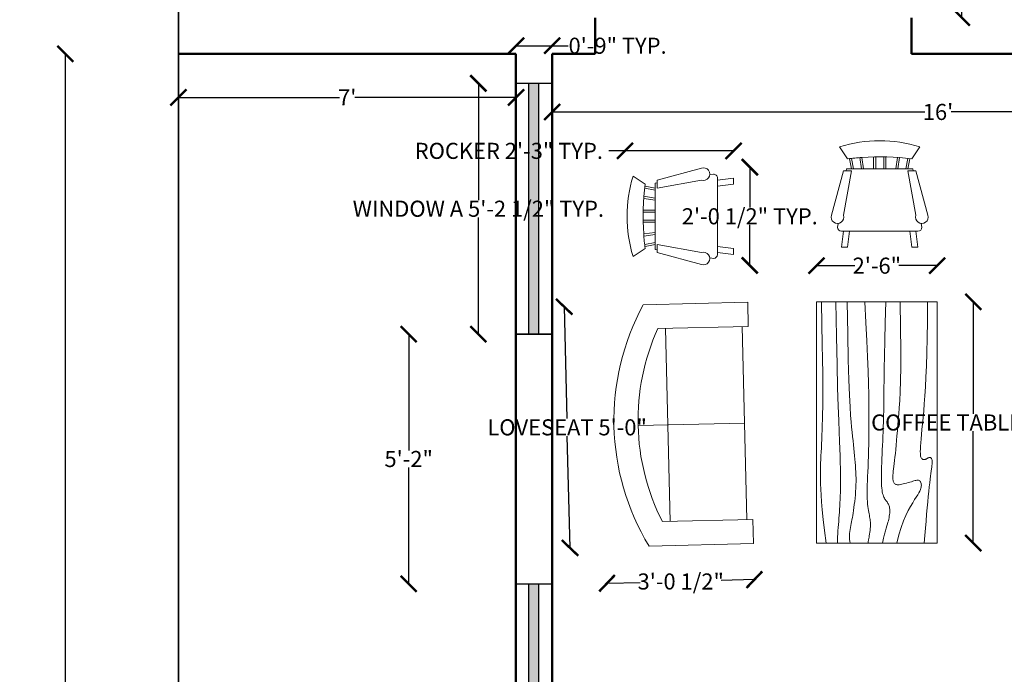
# Model space of a CAD drawing. Units: inches. Extents: x 2466 to 2986, y -30 to 527.
# Tile 2 of 5: x 2466 to 2711, y 190 to 353. Entities that reach past the tile are written whole.
import ezdxf

# ---------------------------------------------------------------- set-up
doc = ezdxf.new("R2010")
doc.units = ezdxf.units.IN
for name, color, linetype, lineweight in [('A-ANNO-DIMS', 2, 'Continuous', 18), ('A-GLAZ', 4, 'Continuous', 25), ('C-PROP', 40, 'Continuous', 35), ('furniture', 6, 'Continuous', 18), ('walls', 40, 'Continuous', 50)]:
    doc.layers.add(name, color=color, linetype=linetype, lineweight=lineweight)
doc.styles.get("Standard").update_dxf_attribs({"font": 'arial.ttf'})
doc.dimstyles.get("Standard").update_dxf_attribs({"dimtxt": 4, "dimasz": 4, "dimexe": 0.18, "dimexo": 0.0625, "dimgap": 0.09, "dimtad": 0, "dimtih": 1, "dimtoh": 1, "dimzin": 0, "dimdsep": 46, "dimlunit": 3, "dimtxsty": 'Standard', "dimblk": 'ARCHTICK', "dimcen": 0.09, "dimse1": 1, "dimse2": 1, "dimclrd": 3, "dimclrt": 2, "dimadec": 0, "dimazin": 0, "dimtfac": 1, "dimtofl": 0, "dimtmove": 0, "dimatfit": 3, "dimfxl": 1, "dimtolj": 1, "dimtzin": 0, "dimarcsym": 0})

# ---------------------------------------------------------------- blocks, each defined once
blk = doc.blocks.new('Sofa - Roundback Loveseat 5 ft.')
for p, q in [((0, -32.44198), (0, -5.99998)), ((-24, -33.99998), (-24, -11.46958)), ((24.00004, -33.99998), (24.00004, -11.46958)), ((-23.9998, -13.38178), (23.99986, -13.38178)), ((-24, -32.44198), (24.00004, -32.44198))]:
    blk.add_line(p, q)
for points in [[(-24, -33.99998), (-30, -33.99998), (-30, -7.99998)], [(30.00004, -7.99998), (30.00004, -33.99998), (24.00004, -33.99998)]]:
    blk.add_lwpolyline(points)
for centre, radius, start, end in [((0, -60.24998), 60.24998, 60.13715, 119.8628), ((0, -61.38438), 55.38444, 64.32083, 115.6792)]:
    blk.add_arc(centre, radius, start, end)
blk = doc.blocks.new('Table - Rectangular Woodgrain 60 x 30 in.')
for p, q in [((0, 0), (0, -30)), ((60, 0), (0, 0)), ((60, -30), (60, 0)), ((0, -30), (60, -30))]:
    blk.add_line(p, q)
for points in [[(0, -2.4), (4.8155, -2.418), (9.0302, -2.4688), (12.709, -2.5477), (15.9167, -2.65), (18.7181, -2.7711), (21.1781, -2.9063), (23.3616, -3.0508), (25.3333, -3.2), (27.1477, -3.3495), (28.8172, -3.4958), (30.3437, -3.636), (31.7291, -3.7667), (32.9756, -3.8849), (34.0849, -3.9875), (35.059, -4.0714), (35.9, -4.1334), (36.6114, -4.1711), (37.2041, -4.1854), (37.6906, -4.1779), (38.0833, -4.15), (38.3948, -4.1034), (38.6375, -4.0396), (38.8239, -3.9602), (38.9666, -3.8667), (39.0764, -3.7608), (39.1573, -3.6448), (39.2116, -3.521), (39.2416, -3.3917), (39.2498, -3.2593), (39.2385, -3.1261), (39.21, -2.9944), (39.1666, -2.8667), (39.111, -2.7447), (39.0468, -2.6281), (38.978, -2.5163), (38.9083, -2.4083), (38.8418, -2.3035), (38.7823, -2.201), (38.7337, -2.1001), (38.7, -2), (38.6844, -1.9003), (38.6875, -1.8021), (38.7094, -1.707), (38.75, -1.6167), (38.8094, -1.5326), (38.8875, -1.4563), (38.9844, -1.3893), (39.1, -1.3333), (39.2351, -1.2896), (39.3937, -1.2583), (39.5804, -1.2396), (39.8, -1.2333), (40.057, -1.2396), (40.3562, -1.2583), (40.7023, -1.2896), (41.1, -1.3333), (41.5547, -1.3895), (42.0755, -1.4573), (42.6721, -1.5361), (43.3542, -1.625), (44.1316, -1.7233), (45.014, -1.8302), (46.0114, -1.9449), (47.1333, -2.0667), (48.3862, -2.1947), (49.7625, -2.3281), (51.2513, -2.4663), (52.8416, -2.6083), (54.5226, -2.7535), (56.2833, -2.9011), (58.1127, -3.0501), (60, -3.2)], [(0, -9.2), (6.5759, -9.0858), (11.9385, -9.0365), (16.2527, -9.0418), (19.6833, -9.0917), (22.3952, -9.1759), (24.5531, -9.2844), (26.322, -9.4069), (27.8666, -9.5333), (29.3241, -9.6553), (30.7203, -9.7719), (32.0532, -9.8837), (33.3208, -9.9917), (34.5213, -10.0965), (35.6526, -10.199), (36.7128, -10.2999), (37.7, -10.4), (38.6129, -10.4996), (39.4531, -10.5969), (40.223, -10.6895), (40.925, -10.775), (41.5613, -10.8512), (42.1344, -10.9156), (42.6465, -10.966), (43.1, -11), (43.4976, -11.0158), (43.8437, -11.0136), (44.143, -10.9942), (44.4, -10.9583), (44.6195, -10.9069), (44.8062, -10.8406), (44.9648, -10.7603), (45.1, -10.6667), (45.2155, -10.5598), (45.3114, -10.4365), (45.3871, -10.2929), (45.4416, -10.125), (45.4743, -9.929), (45.4844, -9.7011), (45.4709, -9.4371), (45.4333, -9.1333), (45.3716, -8.7883), (45.2896, -8.4104), (45.1919, -8.0107), (45.0833, -7.6), (44.9685, -7.1893), (44.8521, -6.7896), (44.7388, -6.4117), (44.6333, -6.0667), (44.54, -5.7628), (44.4614, -5.4979), (44.4001, -5.2675), (44.3583, -5.0667), (44.3384, -4.8909), (44.3427, -4.7354), (44.3736, -4.5956), (44.4333, -4.4667), (44.5236, -4.3453), (44.6427, -4.2333), (44.7884, -4.1339), (44.9583, -4.05), (45.1501, -3.9849), (45.3614, -3.9417), (45.59, -3.9234), (45.8333, -3.9333), (46.0915, -3.9749), (46.3734, -4.0531), (46.6906, -4.1736), (47.0542, -4.3417), (47.4756, -4.5629), (47.9661, -4.8427), (48.5372, -5.1866), (49.2, -5.6), (49.9676, -6.0844), (50.8594, -6.625), (51.8965, -7.2031), (53.1, -7.8), (54.491, -8.3969), (56.0906, -8.975), (57.9199, -9.5156), (60, -10)], [(0, -12.8), (5.1847, -12.9322), (9.6213, -13.0323), (13.3963, -13.1059), (16.5958, -13.1583), (19.3063, -13.1952), (21.614, -13.2219), (23.6054, -13.2439), (25.3666, -13.2667), (26.9728, -13.2947), (28.4531, -13.3281), (29.8256, -13.3663), (31.1083, -13.4083), (32.3191, -13.4535), (33.476, -13.501), (34.597, -13.5501), (35.7, -13.6), (36.7984, -13.6497), (37.8875, -13.6979), (38.9578, -13.743), (40, -13.7833), (41.0047, -13.8174), (41.9625, -13.8438), (42.864, -13.8607), (43.7, -13.8667), (44.4631, -13.8604), (45.1552, -13.8417), (45.7801, -13.8104), (46.3416, -13.7667), (46.8439, -13.7104), (47.2906, -13.6417), (47.6858, -13.5604), (48.0333, -13.4667), (48.3375, -13.3608), (48.6042, -13.2448), (48.8396, -13.121), (49.05, -12.9917), (49.2417, -12.8593), (49.4208, -12.7261), (49.5937, -12.5944), (49.7667, -12.4667), (49.9452, -12.3451), (50.1323, -12.2313), (50.3303, -12.1268), (50.5416, -12.0333), (50.7686, -11.9524), (51.0135, -11.8854), (51.2788, -11.8341), (51.5666, -11.8), (51.8785, -11.7843), (52.2116, -11.7865), (52.562, -11.8059), (52.926, -11.8417), (53.2998, -11.8931), (53.6795, -11.9594), (54.0614, -12.0397), (54.4416, -12.1333), (54.8223, -12.2401), (55.2293, -12.3625), (55.6942, -12.5037), (56.2489, -12.6667), (56.9251, -12.8547), (57.7545, -13.0708), (58.7689, -13.3182), (60, -13.6)], [(0, -18), (5.124, -17.7273), (9.6609, -17.5057), (13.6705, -17.3303), (17.2125, -17.1958), (20.3467, -17.0973), (23.1328, -17.0297), (25.6307, -16.9878), (27.9, -16.9667), (29.9928, -16.9617), (31.9302, -16.9703), (33.7254, -16.9907), (35.3917, -17.0208), (36.9423, -17.0588), (38.3906, -17.1026), (39.7499, -17.1503), (41.0333, -17.2), (42.2519, -17.2496), (43.4073, -17.2969), (44.4986, -17.3395), (45.525, -17.375), (46.4858, -17.4012), (47.3802, -17.4156), (48.2074, -17.416), (48.9667, -17.4), (49.6583, -17.3662), (50.2872, -17.3167), (50.8595, -17.2547), (51.3812, -17.1833), (51.8584, -17.1057), (52.2971, -17.025), (52.7034, -16.9443), (53.0833, -16.8667), (53.443, -16.7951), (53.789, -16.7313), (54.128, -16.6768), (54.4666, -16.6334), (54.8115, -16.6024), (55.1693, -16.5854), (55.5465, -16.5841), (55.95, -16.6), (56.3828, -16.6337), (56.8346, -16.6823), (57.2915, -16.7418), (57.7396, -16.8084), (58.165, -16.878), (58.5539, -16.9469), (58.8924, -17.0111), (59.1666, -17.0667), (59.3679, -17.1107), (59.5078, -17.1438), (59.6032, -17.1675), (59.6708, -17.1833), (59.7275, -17.193), (59.7901, -17.1979), (59.8753, -17.1998), (60, -17.2)], [(0, -22.4), (8.0098, -22.2501), (14.4094, -22.1011), (19.4168, -21.9535), (23.25, -21.8083), (26.1269, -21.6663), (28.2656, -21.5281), (29.884, -21.3947), (31.2, -21.2667), (32.3967, -21.1448), (33.5172, -21.0292), (34.5697, -20.9198), (35.5625, -20.8167), (36.5037, -20.7198), (37.4015, -20.6292), (38.2642, -20.5448), (39.1, -20.4667), (39.9164, -20.3951), (40.7187, -20.3313), (41.5117, -20.2768), (42.3, -20.2333), (43.0883, -20.2024), (43.8812, -20.1854), (44.6836, -20.1841), (45.5, -20.2), (46.3328, -20.234), (47.1747, -20.2844), (48.0163, -20.3488), (48.8479, -20.425), (49.66, -20.5106), (50.4429, -20.6031), (51.1872, -20.7004), (51.8833, -20.8), (52.5246, -20.8999), (53.1166, -20.9995), (53.6681, -21.0983), (54.1875, -21.1958), (54.6834, -21.2919), (55.1646, -21.3859), (55.6394, -21.4777), (56.1167, -21.5667), (56.6028, -21.6515), (57.0961, -21.7266), (57.5929, -21.7852), (58.0896, -21.8208), (58.5823, -21.8268), (59.0674, -21.7964), (59.5412, -21.723), (60, -21.6)], [(0, -25.2), (8.6355, -25.0504), (15.7026, -24.9031), (21.4049, -24.7606), (25.9458, -24.625), (29.529, -24.4988), (32.3578, -24.3844), (34.6359, -24.284), (36.5667, -24.2), (38.3213, -24.1341), (39.9417, -24.0854), (41.437, -24.0523), (42.8167, -24.0333), (44.0901, -24.0268), (45.2667, -24.0313), (46.3557, -24.0451), (47.3667, -24.0667), (48.309, -24.0947), (49.1928, -24.1287), (50.0284, -24.168), (50.826, -24.2125), (51.5959, -24.2617), (52.3483, -24.3151), (53.0935, -24.3725), (53.8417, -24.4334), (54.6009, -24.497), (55.3699, -24.561), (56.1454, -24.6226), (56.9239, -24.6792), (57.7021, -24.7279), (58.4764, -24.7662), (59.2435, -24.7911), (60, -24.8)], [(0, -28.8), (5.6867, -28.6681), (10.45, -28.5698), (14.407, -28.5012), (17.675, -28.4584), (20.3711, -28.4374), (22.6125, -28.4344), (24.5164, -28.4455), (26.2, -28.4667), (27.762, -28.4947), (29.2276, -28.5281), (30.6033, -28.5663), (31.8958, -28.6084), (33.1118, -28.6535), (34.2578, -28.7011), (35.3405, -28.7501), (36.3666, -28.8), (37.3443, -28.8497), (38.288, -28.8974), (39.2137, -28.9412), (40.1375, -28.9792), (41.0753, -29.0093), (42.0432, -29.0297), (43.0572, -29.0384), (44.1333, -29.0333), (45.2936, -29.0114), (46.5843, -28.9641), (48.0579, -28.8816), (49.7666, -28.7542), (51.7629, -28.5721), (54.0989, -28.3255), (56.8272, -28.0048), (60, -27.6)]]:
    blk.add_lwpolyline(points)
blk = doc.blocks.new('Chair - Rocking')
for p, q in [((-8, -4.5), (-10, -1.5)), ((8, -4.5), (10, -1.5)), ((-7.5, -4.5), (-7, -7)), ((-6.5, -7), (-7.02225, -4.43)), ((-4.5, -7), (-4.96674, -4.19951)), ((-4, -7), (-4.40532, -4.16272)), ((-1.5, -4.05012), (-1.5, -7)), ((-1, -7), (-1, -4.05012)), ((1, -7), (1, -4.04655)), ((1.5, -4.05012), (1.5, -7)), ((4, -7), (4.40187, -4.18694)), ((4.5, -7), (4.96761, -4.19437)), ((6.5, -7), (7, -4.4057)), ((7.5, -4.5), (7, -7)), ((-8.23428, -6.99939), (-8.3093, -7.47958)), ((-8.23041, -7), (8.23915, -7)), ((8.31071, -7.48854), (8.23449, -7.00073)), ((-9, -7.5), (-12, -18.49999)), ((-7, -7.5), (-9, -7.5)), ((-9, -18.49999), (-7, -7.5)), ((7, -7.5), (9, -7.5)), ((9, -18.49999), (7, -7.5)), ((9, -7.5), (12, -18.49999)), ((-10.36644, -20.64523), (-10.5, -21.49999)), ((10.5, -21.49999), (10.3575, -20.58798)), ((-9, -22.49999), (-9.5, -26.49999)), ((0, -22.49999), (-9.5, -22.49999)), ((-8, -26.49999), (-7.5, -22.49999)), ((0, -22.49999), (9.5, -22.49999)), ((8, -26.49999), (7.5, -22.49999)), ((9, -22.49999), (9.5, -26.49999)), ((-9.5, -26.49999), (-8, -26.49999)), ((9.5, -26.49999), (8, -26.49999))]:
    blk.add_line(p, q)
for centre, radius, start, end in [((0, -34.08333), 34.08333, 72.93847, 107.0615), ((0, -68.25004), 64.25, 93.92211, 97.15267), ((0, -68.25004), 64.25, 82.84733, 93.92211), ((-10.5, -18.99999), 1.58114, 161.5651, 18.43495), ((10.5, -18.99999), 1.58114, 161.5651, 18.43495), ((-9.5, -21.49999), 1, 180, 270), ((9.5, -21.49999), 1, 270, 0)]:
    blk.add_arc(centre, radius, start, end)
blk = doc.blocks.new('_ArchTick')
at = {"color": 0, "linetype": 'ByBlock', "const_width": 0.15}
blk.add_lwpolyline([(-0.5, -0.5), (0.5, 0.5)], dxfattribs=at)
blk = doc.blocks.new('*D19')
at = {"layer": 'A-ANNO-DIMS', "color": 0, "lineweight": -2, "transparency": 16777216}
for p, q in [((2477.58, 344.8), (2477.58, 174.43)), ((2477.58, -0.2), (2477.58, 170.16))]:
    blk.add_line(p, q, dxfattribs=at)
at = {"layer": 'Defpoints', "color": 0, "transparency": 16777216}
for p in [(2477.58, 344.8), (2505.73, 344.8), (2505.73, -0.2)]:
    blk.add_point(p, dxfattribs=at)
at = {"layer": 'A-ANNO-DIMS', "color": 0, "lineweight": -2, "transparency": 16777216, "xscale": 4, "yscale": 4, "zscale": 4}
for p, rotation in [((2477.58, 344.8), 90), ((2477.58, -0.2), 270)]:
    blk.add_blockref('_ArchTick', p, dxfattribs=dict(at, rotation=rotation))
at = {"layer": 'A-ANNO-DIMS', "color": 0, "transparency": 16777216, "insert": (2477.58, 172.3), "char_height": 4, "attachment_point": 5}
blk.add_mtext('\\A1;28\'-9.00"', dxfattribs=at)
blk = doc.blocks.new('*D20')
at = {"layer": 'A-ANNO-DIMS', "color": 0, "lineweight": -2, "transparency": 16777216}
for p, q in [((2505.73, 333.97), (2545.81, 333.97)), ((2589.73, 333.97), (2549.64, 333.97))]:
    blk.add_line(p, q, dxfattribs=at)
at = {"layer": 'Defpoints', "color": 0, "transparency": 16777216}
for p in [(2505.73, 344.8), (2589.73, 344.8), (2589.73, 333.97)]:
    blk.add_point(p, dxfattribs=at)
at = {"layer": 'A-ANNO-DIMS', "color": 0, "lineweight": -2, "transparency": 16777216, "xscale": 4, "yscale": 4, "zscale": 4, "rotation": 180}
blk.add_blockref('_ArchTick', (2505.73, 333.97), dxfattribs=at)
at = {"layer": 'A-ANNO-DIMS', "color": 0, "lineweight": -2, "transparency": 16777216, "xscale": 4, "yscale": 4, "zscale": 4}
blk.add_blockref('_ArchTick', (2589.73, 333.97), dxfattribs=at)
at = {"layer": 'A-ANNO-DIMS', "color": 0, "transparency": 16777216, "insert": (2547.73, 333.97), "char_height": 4, "attachment_point": 5}
blk.add_mtext("\\A1;7'", dxfattribs=at)
blk = doc.blocks.new('*D25')
at = {"layer": 'A-ANNO-DIMS', "color": 0, "lineweight": -2, "transparency": 16777216}
for p, q in [((2700.63, 485.8), (2700.63, 421.89)), ((2700.63, 353.8), (2700.63, 417.7))]:
    blk.add_line(p, q, dxfattribs=at)
at = {"layer": 'Defpoints', "color": 0, "transparency": 16777216}
for p in [(2706.73, 485.8), (2700.63, 353.8), (2706.73, 353.8)]:
    blk.add_point(p, dxfattribs=at)
at = {"layer": 'A-ANNO-DIMS', "color": 0, "lineweight": -2, "transparency": 16777216, "xscale": 4, "yscale": 4, "zscale": 4}
for p, rotation in [((2700.63, 485.8), 90), ((2700.63, 353.8), 270)]:
    blk.add_blockref('_ArchTick', p, dxfattribs=dict(at, rotation=rotation))
at = {"layer": 'A-ANNO-DIMS', "color": 0, "transparency": 16777216, "insert": (2700.63, 419.8), "char_height": 4, "attachment_point": 5}
blk.add_mtext("\\A1;11'", dxfattribs=at)
blk = doc.blocks.new('*D36')
at = {"layer": 'A-ANNO-DIMS', "color": 0, "lineweight": -2, "transparency": 16777216}
for p, q in [((2598.73, 330.35), (2691.43, 330.35)), ((2790.73, 330.35), (2698.02, 330.35))]:
    blk.add_line(p, q, dxfattribs=at)
at = {"layer": 'Defpoints', "color": 0, "transparency": 16777216}
for p in [(2598.73, 339.99), (2790.73, 339.99), (2598.73, 330.35)]:
    blk.add_point(p, dxfattribs=at)
at = {"layer": 'A-ANNO-DIMS', "color": 0, "lineweight": -2, "transparency": 16777216, "xscale": 4, "yscale": 4, "zscale": 4, "rotation": 180}
blk.add_blockref('_ArchTick', (2598.73, 330.35), dxfattribs=at)
at = {"layer": 'A-ANNO-DIMS', "color": 0, "lineweight": -2, "transparency": 16777216, "xscale": 4, "yscale": 4, "zscale": 4}
blk.add_blockref('_ArchTick', (2790.73, 330.35), dxfattribs=at)
at = {"layer": 'A-ANNO-DIMS', "color": 0, "transparency": 16777216, "insert": (2694.73, 330.35), "char_height": 4, "attachment_point": 5}
blk.add_mtext("\\A1;16'", dxfattribs=at)
blk = doc.blocks.new('WIN-62_38IN')
h = blk.add_hatch(color=256)
h.dxf.hatch_style = 1
h.paths.add_polyline_path([(3.19, 0), (5.61, 0), (5.61, 62.38), (3.19, 62.38)])
for p, q in [((0, 62.38), (9, 62.38)), ((0, 0), (9, 0))]:
    blk.add_line(p, q)
for points in [[(0, 0), (0, 62.38), (9, 62.38), (9, 62.38), (9, 0)], [(3.19, 0), (3.19, 62.38), (5.61, 62.38), (5.61, 0)]]:
    blk.add_lwpolyline(points, close=True)
blk = doc.blocks.new('*D39')
at = {"layer": 'A-ANNO-DIMS', "color": 3, "lineweight": -2, "transparency": 16777216}
for p, q in [((2580.37, 337.46), (2580.37, 308.43)), ((2580.37, 275.09), (2580.37, 304.12))]:
    blk.add_line(p, q, dxfattribs=at)
at = {"layer": 'Defpoints', "color": 0, "transparency": 16777216}
for p in [(2580.37, 337.46), (2589.73, 337.46), (2589.73, 275.09)]:
    blk.add_point(p, dxfattribs=at)
at = {"layer": 'A-ANNO-DIMS', "color": 3, "lineweight": -2, "transparency": 16777216, "xscale": 4, "yscale": 4, "zscale": 4}
for p, rotation in [((2580.37, 337.46), 90), ((2580.37, 275.09), 270)]:
    blk.add_blockref('_ArchTick', p, dxfattribs=dict(at, rotation=rotation))
at = {"layer": 'A-ANNO-DIMS', "color": 2, "transparency": 16777216, "insert": (2580.37, 306.28), "char_height": 4, "attachment_point": 5}
blk.add_mtext('\\A1;WINDOW A 5\'-2 1/2" TYP.', dxfattribs=at)
blk = doc.blocks.new('*D40')
at = {"layer": 'A-ANNO-DIMS', "color": 3, "lineweight": -2, "transparency": 16777216}
for p, q in [((2589.73, 346.82), (2598.73, 346.82)), ((2598.73, 346.82), (2602.73, 346.82))]:
    blk.add_line(p, q, dxfattribs=at)
at = {"layer": 'Defpoints', "color": 0, "transparency": 16777216}
for p in [(2598.73, 346.82), (2589.73, 337.46), (2598.73, 337.46)]:
    blk.add_point(p, dxfattribs=at)
at = {"layer": 'A-ANNO-DIMS', "color": 3, "lineweight": -2, "transparency": 16777216, "xscale": 4, "yscale": 4, "zscale": 4, "rotation": 180}
blk.add_blockref('_ArchTick', (2589.73, 346.82), dxfattribs=at)
at = {"layer": 'A-ANNO-DIMS', "color": 3, "lineweight": -2, "transparency": 16777216, "xscale": 4, "yscale": 4, "zscale": 4}
blk.add_blockref('_ArchTick', (2598.73, 346.82), dxfattribs=at)
at = {"layer": 'A-ANNO-DIMS', "color": 2, "transparency": 16777216, "insert": (2615.01, 346.82), "char_height": 4, "attachment_point": 5}
blk.add_mtext('\\A1;0\'-9" TYP.', dxfattribs=at)
blk = doc.blocks.new('*D49')
at = {"layer": 'A-ANNO-DIMS', "color": 3, "lineweight": -2, "transparency": 16777216}
for p, q in [((2616.85, 320.67), (2612.85, 320.67)), ((2643.85, 320.67), (2616.85, 320.67))]:
    blk.add_line(p, q, dxfattribs=at)
at = {"layer": 'Defpoints', "color": 0, "transparency": 16777216}
for p in [(2616.85, 320.67), (2616.85, 316.62), (2643.85, 316.62)]:
    blk.add_point(p, dxfattribs=at)
at = {"layer": 'A-ANNO-DIMS', "color": 3, "lineweight": -2, "transparency": 16777216, "xscale": 4, "yscale": 4, "zscale": 4, "rotation": 180}
blk.add_blockref('_ArchTick', (2616.85, 320.67), dxfattribs=at)
at = {"layer": 'A-ANNO-DIMS', "color": 3, "lineweight": -2, "transparency": 16777216, "xscale": 4, "yscale": 4, "zscale": 4}
blk.add_blockref('_ArchTick', (2643.85, 320.67), dxfattribs=at)
at = {"layer": 'A-ANNO-DIMS', "color": 2, "transparency": 16777216, "insert": (2587.95, 320.67), "char_height": 4, "attachment_point": 5}
blk.add_mtext('\\A1;ROCKER 2\'-3" TYP.', dxfattribs=at)
blk = doc.blocks.new('*D50')
at = {"layer": 'A-ANNO-DIMS', "color": 3, "lineweight": -2, "transparency": 16777216}
for p, q in [((2647.9, 316.62), (2647.9, 306.56)), ((2647.9, 292.18), (2647.9, 302.24))]:
    blk.add_line(p, q, dxfattribs=at)
at = {"layer": 'Defpoints', "color": 0, "transparency": 16777216}
for p in [(2643.85, 316.62), (2647.9, 316.62), (2643.85, 292.18)]:
    blk.add_point(p, dxfattribs=at)
at = {"layer": 'A-ANNO-DIMS', "color": 3, "lineweight": -2, "transparency": 16777216, "xscale": 4, "yscale": 4, "zscale": 4}
for p, rotation in [((2647.9, 316.62), 90), ((2647.9, 292.18), 270)]:
    blk.add_blockref('_ArchTick', p, dxfattribs=dict(at, rotation=rotation))
at = {"layer": 'A-ANNO-DIMS', "color": 2, "transparency": 16777216, "insert": (2647.9, 304.4), "char_height": 4, "attachment_point": 5}
blk.add_mtext('\\A1;2\'-0 1/2" TYP.', dxfattribs=at)
blk = doc.blocks.new('*D55')
at = {"layer": 'A-ANNO-DIMS', "color": 3, "lineweight": -2, "transparency": 16777216}
for p, q in [((2601.72, 281.9), (2602.4, 254.07)), ((2603.17, 221.92), (2602.5, 249.75))]:
    blk.add_line(p, q, dxfattribs=at)
at = {"layer": 'Defpoints', "color": 0, "transparency": 16777216}
for p in [(2601.72, 281.9), (2610.72, 282.12), (2612.17, 222.14)]:
    blk.add_point(p, dxfattribs=at)
at = {"layer": 'A-ANNO-DIMS', "color": 3, "lineweight": -2, "transparency": 16777216, "xscale": 4, "yscale": 4, "zscale": 4}
for p, rotation in [((2601.72, 281.9), 91.3839546849317), ((2603.17, 221.92), 271.3839546849317)]:
    blk.add_blockref('_ArchTick', p, dxfattribs=dict(at, rotation=rotation))
at = {"layer": 'A-ANNO-DIMS', "color": 2, "transparency": 16777216, "insert": (2602.45, 251.91), "char_height": 4, "attachment_point": 5}
blk.add_mtext('\\A1;LOVESEAT 5\'-0"', dxfattribs=at)
blk = doc.blocks.new('*D56')
at = {"layer": 'A-ANNO-DIMS', "color": 3, "lineweight": -2, "transparency": 16777216}
for p, q in [((2612.39, 213.14), (2620.65, 213.34)), ((2649.04, 214.03), (2640.78, 213.83))]:
    blk.add_line(p, q, dxfattribs=at)
at = {"layer": 'Defpoints', "color": 0, "transparency": 16777216}
for p in [(2648.83, 223.02), (2612.17, 222.14), (2612.39, 213.14)]:
    blk.add_point(p, dxfattribs=at)
at = {"layer": 'A-ANNO-DIMS', "color": 3, "lineweight": -2, "transparency": 16777216, "xscale": 4, "yscale": 4, "zscale": 4}
for p, rotation in [((2649.04, 214.03), 1.383954684931536), ((2612.39, 213.14), 181.3839546849315)]:
    blk.add_blockref('_ArchTick', p, dxfattribs=dict(at, rotation=rotation))
at = {"layer": 'A-ANNO-DIMS', "color": 2, "transparency": 16777216, "insert": (2630.72, 213.58), "char_height": 4, "attachment_point": 5}
blk.add_mtext('\\A1;3\'-0 1/2"', dxfattribs=at)
blk = doc.blocks.new('*D57')
at = {"layer": 'A-ANNO-DIMS', "color": 3, "lineweight": -2, "transparency": 16777216}
for p, q in [((2703.51, 283.12), (2703.51, 255.28)), ((2703.51, 223.12), (2703.51, 250.96))]:
    blk.add_line(p, q, dxfattribs=at)
at = {"layer": 'Defpoints', "color": 0, "transparency": 16777216}
for p in [(2694.51, 283.12), (2694.51, 223.12), (2703.51, 223.12)]:
    blk.add_point(p, dxfattribs=at)
at = {"layer": 'A-ANNO-DIMS', "color": 3, "lineweight": -2, "transparency": 16777216, "xscale": 4, "yscale": 4, "zscale": 4}
for p, rotation in [((2703.51, 283.12), 90), ((2703.51, 223.12), 270)]:
    blk.add_blockref('_ArchTick', p, dxfattribs=dict(at, rotation=rotation))
at = {"layer": 'A-ANNO-DIMS', "color": 2, "transparency": 16777216, "insert": (2703.51, 253.12), "char_height": 4, "attachment_point": 5}
blk.add_mtext('\\A1;COFFEE TABLE 5\'-0"', dxfattribs=at)
blk = doc.blocks.new('*D58')
at = {"layer": 'A-ANNO-DIMS', "color": 3, "lineweight": -2, "transparency": 16777216}
for p, q in [((2664.51, 292.12), (2674.07, 292.12)), ((2694.51, 292.12), (2684.95, 292.12))]:
    blk.add_line(p, q, dxfattribs=at)
at = {"layer": 'Defpoints', "color": 0, "transparency": 16777216}
for p in [(2694.51, 292.12), (2664.51, 283.12), (2694.51, 283.12)]:
    blk.add_point(p, dxfattribs=at)
at = {"layer": 'A-ANNO-DIMS', "color": 3, "lineweight": -2, "transparency": 16777216, "xscale": 4, "yscale": 4, "zscale": 4, "rotation": 180}
blk.add_blockref('_ArchTick', (2664.51, 292.12), dxfattribs=at)
at = {"layer": 'A-ANNO-DIMS', "color": 3, "lineweight": -2, "transparency": 16777216, "xscale": 4, "yscale": 4, "zscale": 4}
blk.add_blockref('_ArchTick', (2694.51, 292.12), dxfattribs=at)
at = {"layer": 'A-ANNO-DIMS', "color": 2, "transparency": 16777216, "insert": (2679.51, 292.12), "char_height": 4, "attachment_point": 5}
blk.add_mtext('\\A1;2\'-6"', dxfattribs=at)
blk = doc.blocks.new('*D75')
at = {"layer": 'A-ANNO-DIMS', "color": 3, "lineweight": -2, "transparency": 16777216}
for p, q in [((2563.03, 275.09), (2563.03, 246.17)), ((2563.03, 212.99), (2563.03, 241.9))]:
    blk.add_line(p, q, dxfattribs=at)
at = {"layer": 'Defpoints', "color": 0, "transparency": 16777216}
for p in [(2563.03, 275.09), (2589.73, 275.09), (2589.73, 212.99)]:
    blk.add_point(p, dxfattribs=at)
at = {"layer": 'A-ANNO-DIMS', "color": 3, "lineweight": -2, "transparency": 16777216, "xscale": 4, "yscale": 4, "zscale": 4}
for p, rotation in [((2563.03, 275.09), 90), ((2563.03, 212.99), 270)]:
    blk.add_blockref('_ArchTick', p, dxfattribs=dict(at, rotation=rotation))
at = {"layer": 'A-ANNO-DIMS', "color": 2, "transparency": 16777216, "insert": (2563.03, 244.04), "char_height": 4, "attachment_point": 5}
blk.add_mtext('\\A1;5\'-2"', dxfattribs=at)

msp = doc.modelspace()

# ---------------------------------------------------------------- linework, layer by layer
at = {"layer": 'C-PROP'}
msp.add_line((2505.725, 494.795), (2505.725, -0.205), dxfattribs=at)
at = {"layer": 'walls'}
for p, q in [((2609.399, 353.795), (2609.399, 344.795)), ((2688.139, 353.795), (2688.139, 344.795)), ((2505.725, 344.795), (2589.725, 344.795)), ((2589.725, 344.795), (2589.725, 131.795)), ((2598.725, 344.795), (2598.725, 140.795)), ((2598.725, 344.795), (2609.399, 344.795)), ((2688.139, 344.795), (2721.753, 344.795))]:
    msp.add_line(p, q, dxfattribs=at)

# ---------------------------------------------------------------- block references
at = {"layer": 'A-GLAZ'}
for p in [(2589.725, 275.086), (2589.725, 150.606)]:
    msp.add_blockref('WIN-62_38IN', p, dxfattribs=at)
at = {"layer": 'furniture'}
msp.add_blockref('Chair - Rocking', (2680.221, 323.187), dxfattribs=at)
for name, p, rotation in [('Chair - Rocking', (2617.355, 304.4), 90.00000000000003), ('Sofa - Roundback Loveseat 5 ft.', (2614.113, 252.195), 91.3839546849315), ('Table - Rectangular Woodgrain 60 x 30 in.', (2694.512, 283.123), 270)]:
    msp.add_blockref(name, p, dxfattribs=dict(at, rotation=rotation))

# ---------------------------------------------------------------- dimensions: what is measured, and where the dimension line sits
at = {"layer": 'A-ANNO-DIMS'}
for base, p1, p2, angle, override, picture, middle in [((2700.632, 353.795), (2706.725, 485.795), (2706.725, 353.795), 90, {"dimclrd": 0, "dimclre": 0, "dimclrt": 0}, '*D25', (2700.632, 419.795)), ((2477.576, 344.795), (2505.725, -0.205), (2505.725, 344.795), 90, {"dimclrd": 0, "dimclre": 0, "dimclrt": 0}, '*D19', (2477.576, 172.295)), ((2563.025, 275.086), (2589.725, 212.985), (2589.725, 275.086), 90, {"dimdec": 1, "dimlfac": 1, "dimrnd": 0, "dimzin": 1, "dimdsep": 46, "dimlunit": 4, "dimfrac": 2}, '*D75', (2563.025, 244.036)), ((2612.389, 213.142), (2648.827, 223.025), (2612.171, 222.139), 181.38395, {"dimdec": 1, "dimlfac": 1, "dimrnd": 0, "dimzin": 1, "dimdsep": 46, "dimlunit": 4, "dimfrac": 2}, '*D56', (2630.717, 213.584))]:
    dim = msp.add_linear_dim(base=base, p1=p1, p2=p2, angle=angle, dimstyle='Standard', override=override, dxfattribs=at)
    dim.commit()
    dim.dimension.update_dxf_attribs({"geometry": picture, "text_midpoint": middle})
dim = msp.add_linear_dim(base=(2598.725, 346.822), p1=(2589.725, 337.465), p2=(2598.725, 337.465), text='<> TYP.', dimstyle='Standard', override={"dimdec": 1, "dimlfac": 1, "dimrnd": 0, "dimzin": 1, "dimdsep": 46, "dimlunit": 4, "dimfrac": 2}, dxfattribs=at)
dim.commit()
dim.dimension.update_dxf_attribs({"geometry": '*D40', "text_midpoint": (2615.006, 346.822)})
for base, p1, p2, override, picture, middle in [((2589.725, 333.966), (2505.725, 344.795), (2589.725, 344.795), {"dimclrd": 0, "dimclre": 0, "dimclrt": 0}, '*D20', (2547.725, 333.966)), ((2598.725, 330.35), (2790.725, 339.988), (2598.725, 339.988), {"dimclrd": 0, "dimclre": 0, "dimclrt": 0}, '*D36', (2694.725, 330.35)), ((2694.512, 292.123), (2664.512, 283.123), (2694.512, 283.123), {"dimdec": 1, "dimlfac": 1, "dimrnd": 0, "dimzin": 1, "dimdsep": 46, "dimlunit": 4, "dimfrac": 2}, '*D58', (2679.512, 292.123))]:
    dim = msp.add_linear_dim(base=base, p1=p1, p2=p2, dimstyle='Standard', override=override, dxfattribs=at)
    dim.commit()
    dim.dimension.update_dxf_attribs({"geometry": picture, "text_midpoint": middle})
for base, p1, p2, angle, text, picture, middle in [((2580.369, 337.465), (2589.725, 275.086), (2589.725, 337.465), 90, 'WINDOW A <> TYP.', '*D39', (2580.369, 306.275)), ((2616.855, 320.668), (2643.855, 316.618), (2616.855, 316.618), 180, 'ROCKER <> TYP.', '*D49', (2587.948, 320.668)), ((2647.905, 316.618), (2643.855, 292.183), (2643.855, 316.618), 90, '<> TYP.', '*D50', (2647.905, 304.4)), ((2703.512, 223.123), (2694.512, 283.123), (2694.512, 223.123), 270, 'COFFEE TABLE <>', '*D57', (2703.512, 253.123)), ((2601.725, 281.904), (2612.171, 222.139), (2610.722, 282.122), 91.38395, 'LOVESEAT <>', '*D55', (2602.449, 251.913))]:
    dim = msp.add_linear_dim(base=base, p1=p1, p2=p2, angle=angle, text=text, dimstyle='Standard', override={"dimdec": 1, "dimlfac": 1, "dimrnd": 0, "dimzin": 1, "dimdsep": 46, "dimlunit": 4, "dimfrac": 2}, dxfattribs=at)
    dim.commit()
    dim.dimension.update_dxf_attribs({"geometry": picture, "text_midpoint": middle})

doc.saveas('drawing.dxf')
